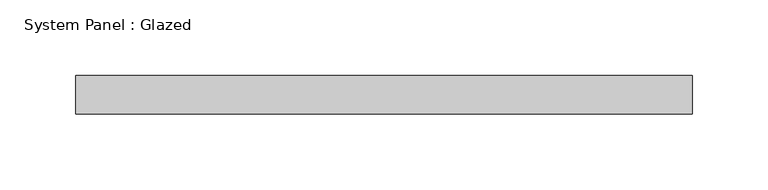
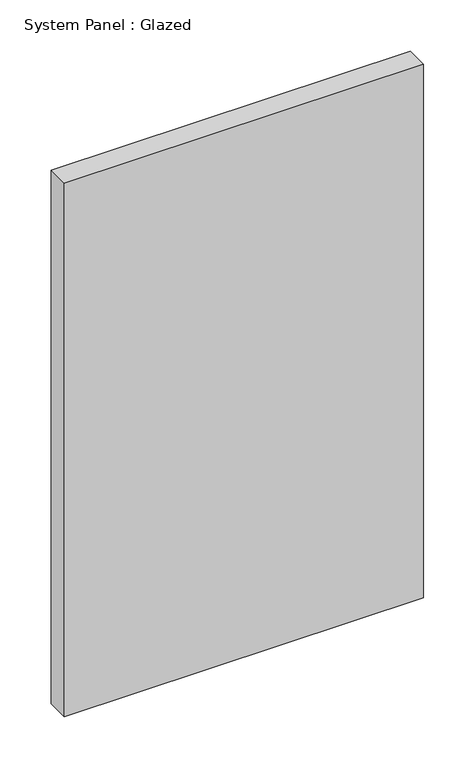
"""IFC4 building model written with IfcOpenShell, lengths in millimetres: plate geometry, System Panel : Glazed."""

from ifc_helpers import new_model, si_unit, origin, origin_with_axes, place, context, project, spatial, polyline, outline, extrude, source, transform, mapped, element, save


def system_panel_glazed_0c192b01(model_context):
    return source(origin(), model_context, "Body", "SweptSolid", [
        extrude(outline(polyline([(203.2, 19.05), (-203.2, 19.05), (-203.2, 44.45), (203.2, 44.45), (203.2, 19.05)])), origin_with_axes(), (0.0, 0.0, 1.0), 637.2305927),
    ])


if __name__ == "__main__":
    model = new_model("IFC4")
    model_context = context("Model", 3, world=origin())
    ifc_project = project(units=[si_unit("LENGTHUNIT", "METRE", prefix="MILLI")], contexts=[model_context])
    site = spatial("IfcSite", under=ifc_project)
    building = spatial("IfcBuilding", under=site)
    placement = place(None, origin())
    system_panel_glazed_shape = system_panel_glazed_0c192b01(model_context)
    element("IfcPlate", 1, ObjectType="System Panel : Glazed", at=placement, inside=building, context=model_context, shape_type="MappedRepresentation", body=[
        mapped(system_panel_glazed_shape, transform((0.0, 0.0, 0.0), x_axis=(1.0, 0.0, 0.0), y_axis=(0.0, 1.0, 0.0), z_axis=(0.0, 0.0, 1.0))),
    ])
    save(model, "model.ifc")

# Revit data of these elements
# Type "System Panel : Glazed"
#   Construction Type Id = "GSP4R"
#   Analytic Construction = "1/8 in Pilkington single glazing"
#   Visual Light Transmittance = 0.9
#   Solar Heat Gain Coefficient = 0.86
#   Heat Transfer Coefficient (U) = 1.18115 BTU/(h·ft²·°F)
#   Define Thermal Properties by = 1
# Element 1 (IfcPlate, "System Panel : Glazed")
#   Materials on its faces: "Glass"
# Materials
#   "Glass": class "Glass", colour RGB 0 128 192, transparency 0.75, Description = "Soda Lime Glass", Cost = 0
